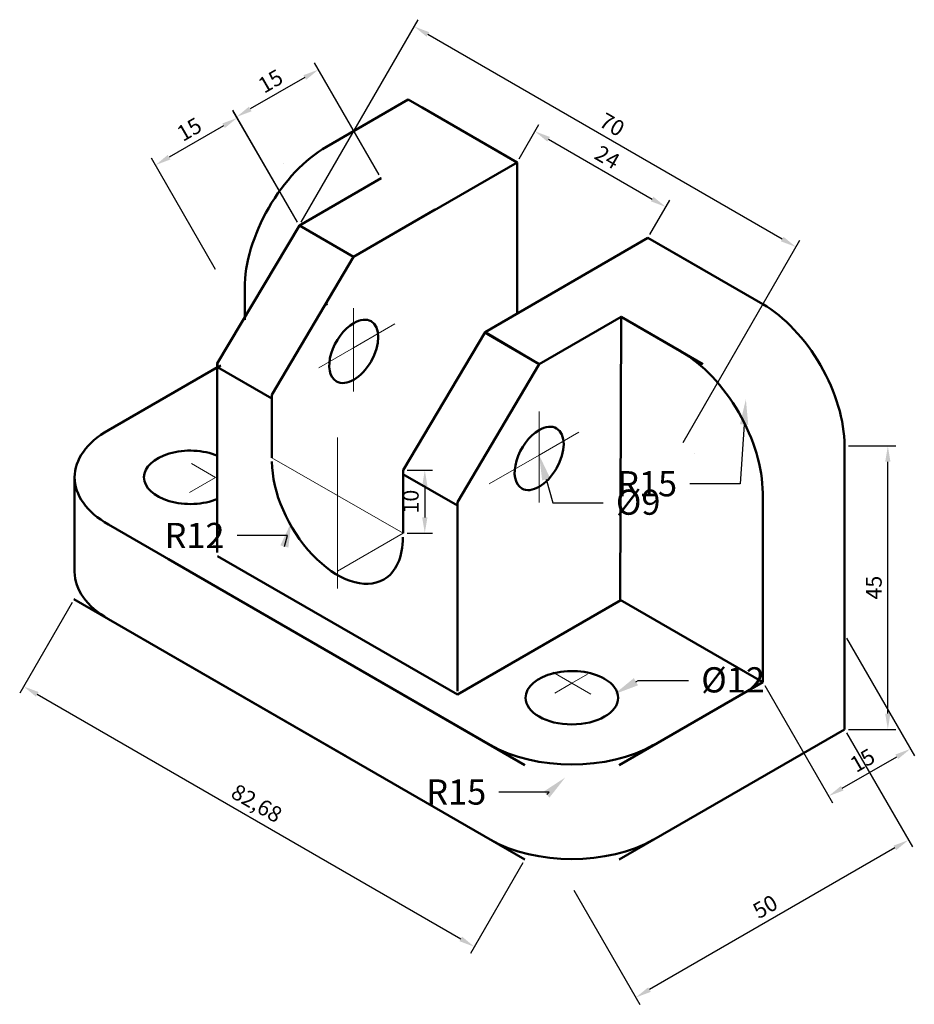
# Model space of a CAD drawing. Units: millimetres. Extents: x 2245 to 2387, y 1433 to 1590.
import ezdxf
from ezdxf import colors
from ezdxf.entities.mleader import LeaderData, LeaderLine
from ezdxf.math import Vec2, Vec3

# ---------------------------------------------------------------- set-up
doc = ezdxf.new("R2010")
doc.units = ezdxf.units.MM
doc.linetypes.add('CENTER', pattern=[50.8, 31.75, -6.35, 6.35, -6.35])
for name, color, linetype, lineweight in [('M-CNTR', 4, 'CENTER', 18), ('M-DIMS', 2, 'Continuous', 25), ('M-OUTL', 7, 'Continuous', 50)]:
    doc.layers.add(name, color=color, linetype=linetype, lineweight=lineweight)
doc.styles.get("Standard").update_dxf_attribs({"font": 'arial.ttf'})
doc.dimstyles.new('ISO-25', dxfattribs={"dimtxt": 2.5, "dimasz": 2.5, "dimexe": 1.25, "dimexo": 0.625, "dimtad": 1, "dimtxsty": 'Standard', "dimcen": 2.5, "dimadec": 0, "dimazin": 0, "dimtfac": 1, "dimtmove": 0, "dimatfit": 3, "dimfxl": 1, "dimarcsym": 0})

# ---------------------------------------------------------------- blocks, each defined once
blk = doc.blocks.new('*D1')
at = {"layer": 'Defpoints', "color": 0, "transparency": 16777216}
for p in [(2324.24, 1567.07), (2347.86, 1559.99), (2345.02, 1555.07)]:
    blk.add_point(p, dxfattribs=at)
at = {"layer": 'M-DIMS', "color": 0, "lineweight": -2, "transparency": 16777216}
for p, q in [((2324.55, 1567.61), (2327.7, 1573.07)), ((2329.24, 1570.74), (2345.69, 1561.24)), ((2345.33, 1555.61), (2348.48, 1561.07))]:
    blk.add_line(p, q, dxfattribs=at)
at = {"layer": 'M-DIMS', "color": 0, "transparency": 16777216}
for points in [[(2329.45, 1571.1), (2329.03, 1570.38), (2327.08, 1571.99)], [(2345.9, 1561.6), (2345.49, 1560.88), (2347.86, 1559.99)]]:
    blk.add_solid(points, dxfattribs=at)
at = {"layer": 'M-DIMS', "color": 0, "transparency": 16777216, "insert": (2338.41, 1567.62), "char_height": 2.5, "attachment_point": 5, "rotation": 330}
blk.add_mtext('24', dxfattribs=at)
blk = doc.blocks.new('*D2')
at = {"layer": 'Defpoints', "color": 0, "transparency": 16777216}
for p in [(2307.9, 1588.64), (2289.65, 1557.04), (2350.27, 1522.04)]:
    blk.add_point(p, dxfattribs=at)
at = {"layer": 'M-DIMS', "color": 0, "lineweight": -2, "transparency": 16777216}
for p, q in [((2289.96, 1557.58), (2308.52, 1589.73)), ((2366.35, 1554.89), (2310.06, 1587.39)), ((2350.59, 1522.58), (2369.14, 1554.73))]:
    blk.add_line(p, q, dxfattribs=at)
at = {"layer": 'M-DIMS', "color": 0, "transparency": 16777216}
for points in [[(2310.27, 1587.75), (2309.85, 1587.03), (2307.9, 1588.64)], [(2366.56, 1555.25), (2366.15, 1554.53), (2368.52, 1553.64)]]:
    blk.add_solid(points, dxfattribs=at)
at = {"layer": 'M-DIMS', "color": 0, "transparency": 16777216, "insert": (2339.16, 1572.79), "char_height": 2.5, "attachment_point": 5, "rotation": 330}
blk.add_mtext('70', dxfattribs=at)
blk = doc.blocks.new('*D3')
at = {"layer": 'Defpoints', "color": 0, "transparency": 16777216}
for p in [(2376.25, 1522.04), (2383.12, 1522.04), (2376.25, 1477.04)]:
    blk.add_point(p, dxfattribs=at)
at = {"layer": 'M-DIMS', "color": 0, "lineweight": -2, "transparency": 16777216}
for p, q in [((2376.88, 1522.04), (2384.37, 1522.04)), ((2383.12, 1479.54), (2383.12, 1519.54)), ((2376.88, 1477.04), (2384.37, 1477.04))]:
    blk.add_line(p, q, dxfattribs=at)
at = {"layer": 'M-DIMS', "color": 0, "transparency": 16777216}
for points in [[(2382.7, 1519.54), (2383.54, 1519.54), (2383.12, 1522.04)], [(2382.7, 1479.54), (2383.54, 1479.54), (2383.12, 1477.04)]]:
    blk.add_solid(points, dxfattribs=at)
at = {"layer": 'M-DIMS', "color": 0, "transparency": 16777216, "insert": (2381.22, 1499.54), "char_height": 2.5, "attachment_point": 5, "rotation": 90}
blk.add_mtext('45', dxfattribs=at)
blk = doc.blocks.new('*D4')
at = {"layer": 'Defpoints', "color": 0, "transparency": 16777216}
for p in [(2376.25, 1492.04), (2363.26, 1484.54), (2386.7, 1473.94)]:
    blk.add_point(p, dxfattribs=at)
at = {"layer": 'M-DIMS', "color": 0, "lineweight": -2, "transparency": 16777216}
for p, q in [((2376.57, 1491.5), (2387.33, 1472.86)), ((2363.58, 1484), (2374.34, 1465.36)), ((2375.88, 1467.69), (2384.54, 1472.69))]:
    blk.add_line(p, q, dxfattribs=at)
at = {"layer": 'M-DIMS', "color": 0, "transparency": 16777216}
for points in [[(2384.33, 1473.05), (2384.75, 1472.33), (2386.7, 1473.94)], [(2375.67, 1468.05), (2376.08, 1467.33), (2373.71, 1466.44)]]:
    blk.add_solid(points, dxfattribs=at)
at = {"layer": 'M-DIMS', "color": 0, "transparency": 16777216, "insert": (2379.26, 1471.84), "char_height": 2.5, "attachment_point": 5, "rotation": 30}
blk.add_mtext('15', dxfattribs=at)
blk = doc.blocks.new('*D5')
at = {"layer": 'Defpoints', "color": 0, "transparency": 16777216}
for p in [(2376.25, 1477.04), (2332.95, 1452.04), (2343.1, 1434.47)]:
    blk.add_point(p, dxfattribs=at)
at = {"layer": 'M-DIMS', "color": 0, "lineweight": -2, "transparency": 16777216}
for p, q in [((2376.57, 1476.5), (2387.02, 1458.38)), ((2384.23, 1458.22), (2345.26, 1435.72)), ((2333.26, 1451.5), (2343.72, 1433.38))]:
    blk.add_line(p, q, dxfattribs=at)
at = {"layer": 'M-DIMS', "color": 0, "transparency": 16777216}
for points in [[(2384.02, 1458.58), (2384.44, 1457.86), (2386.4, 1459.47)], [(2345.05, 1436.08), (2345.47, 1435.36), (2343.1, 1434.47)]]:
    blk.add_solid(points, dxfattribs=at)
at = {"layer": 'M-DIMS', "color": 0, "transparency": 16777216, "insert": (2363.8, 1448.61), "char_height": 2.5, "attachment_point": 5, "rotation": 30}
blk.add_mtext('50', dxfattribs=at)
blk = doc.blocks.new('*D6')
at = {"layer": 'Defpoints', "color": 0, "transparency": 16777216}
for p in [(2279.69, 1574.3), (2302.64, 1564.54), (2289.65, 1557.04)]:
    blk.add_point(p, dxfattribs=at)
at = {"layer": 'M-DIMS', "color": 0, "lineweight": -2, "transparency": 16777216}
for p, q in [((2302.33, 1565.08), (2292.05, 1582.88)), ((2290.51, 1580.55), (2281.85, 1575.55)), ((2289.34, 1557.58), (2279.06, 1575.38))]:
    blk.add_line(p, q, dxfattribs=at)
at = {"layer": 'M-DIMS', "color": 0, "transparency": 16777216}
for points in [[(2290.3, 1580.91), (2290.72, 1580.18), (2292.68, 1581.8)], [(2281.64, 1575.91), (2282.06, 1575.18), (2279.69, 1574.3)]]:
    blk.add_solid(points, dxfattribs=at)
at = {"layer": 'M-DIMS', "color": 0, "transparency": 16777216, "insert": (2285.23, 1579.69), "char_height": 2.5, "attachment_point": 5, "rotation": 30}
blk.add_mtext('15', dxfattribs=at)
blk = doc.blocks.new('*D7')
at = {"layer": 'Defpoints', "color": 0, "transparency": 16777216}
for p in [(2266.79, 1566.64), (2289.65, 1557.04), (2276.66, 1549.54)]:
    blk.add_point(p, dxfattribs=at)
at = {"layer": 'M-DIMS', "color": 0, "lineweight": -2, "transparency": 16777216}
for p, q in [((2289.34, 1557.58), (2279.15, 1575.22)), ((2277.61, 1572.89), (2268.95, 1567.89)), ((2276.35, 1550.08), (2266.16, 1567.72))]:
    blk.add_line(p, q, dxfattribs=at)
at = {"layer": 'M-DIMS', "color": 0, "transparency": 16777216}
for points in [[(2277.41, 1573.25), (2277.82, 1572.53), (2279.78, 1574.14)], [(2268.74, 1568.25), (2269.16, 1567.53), (2266.79, 1566.64)]]:
    blk.add_solid(points, dxfattribs=at)
at = {"layer": 'M-DIMS', "color": 0, "transparency": 16777216, "insert": (2272.33, 1572.04), "char_height": 2.5, "attachment_point": 5, "rotation": 30}
blk.add_mtext('15', dxfattribs=at)
blk = doc.blocks.new('*D8')
at = {"layer": 'Defpoints', "color": 0, "transparency": 16777216}
for p in [(2306.16, 1518.2), (2306.16, 1508.2), (2309.57, 1508.2)]:
    blk.add_point(p, dxfattribs=at)
at = {"layer": 'M-DIMS', "color": 0, "lineweight": -2, "transparency": 16777216}
for p, q in [((2306.79, 1518.2), (2310.82, 1518.2)), ((2309.57, 1515.7), (2309.57, 1510.7)), ((2306.79, 1508.2), (2310.82, 1508.2))]:
    blk.add_line(p, q, dxfattribs=at)
at = {"layer": 'M-DIMS', "color": 0, "transparency": 16777216}
for points in [[(2309.16, 1515.7), (2309.99, 1515.7), (2309.57, 1518.2)], [(2309.16, 1510.7), (2309.99, 1510.7), (2309.57, 1508.2)]]:
    blk.add_solid(points, dxfattribs=at)
at = {"layer": 'M-DIMS', "color": 0, "transparency": 16777216, "insert": (2307.67, 1513.2), "char_height": 2.5, "attachment_point": 5, "rotation": 90}
blk.add_mtext('10', dxfattribs=at)
blk = doc.blocks.new('*D9')
at = {"layer": 'Defpoints', "color": 0, "transparency": 16777216}
for p in [(2253.85, 1497.71), (2325.45, 1456.37), (2317.45, 1442.52)]:
    blk.add_point(p, dxfattribs=at)
at = {"layer": 'M-DIMS', "color": 0, "lineweight": -2, "transparency": 16777216}
for p, q in [((2253.54, 1497.17), (2245.23, 1482.77)), ((2248.02, 1482.61), (2315.29, 1443.77)), ((2325.14, 1455.83), (2316.83, 1441.43))]:
    blk.add_line(p, q, dxfattribs=at)
at = {"layer": 'M-DIMS', "color": 0, "transparency": 16777216}
for points in [[(2248.23, 1482.97), (2247.81, 1482.24), (2245.85, 1483.86)], [(2315.5, 1444.13), (2315.08, 1443.4), (2317.45, 1442.52)]]:
    blk.add_solid(points, dxfattribs=at)
at = {"layer": 'M-DIMS', "color": 0, "transparency": 16777216, "insert": (2282.72, 1465.03), "char_height": 2.5, "attachment_point": 5, "rotation": 330}
blk.add_mtext('82,68', dxfattribs=at)

msp = doc.modelspace()

# ---------------------------------------------------------------- linework, layer by layer
at = {"layer": 'M-CNTR'}
for p, q in [((2298.237, 1537.629), (2298.237, 1543.93)), ((2298.237, 1537.629), (2304.814, 1541.426)), ((2298.237, 1537.629), (2292.726, 1534.447)), ((2298.237, 1537.629), (2298.237, 1530.715)), ((2327.737, 1520.597), (2327.737, 1527.487)), ((2295.714, 1514.172), (2295.714, 1523.41)), ((2327.737, 1520.597), (2334.016, 1524.222)), ((2285.266, 1520.139), (2306.162, 1508.204)), ((2327.737, 1520.597), (2319.789, 1516.008)), ((2327.737, 1520.597), (2327.737, 1513.074)), ((2276.35, 1517.039), (2272.538, 1519.239)), ((2276.35, 1517.039), (2272.204, 1514.645)), ((2295.714, 1514.172), (2295.714, 1499.42)), ((2295.714, 1502.172), (2306.162, 1508.204)), ((2332.952, 1484.359), (2329.927, 1486.106)), ((2332.952, 1484.359), (2335.435, 1485.793)), ((2332.952, 1484.359), (2330.227, 1482.786)), ((2332.952, 1484.359), (2335.951, 1482.628))]:
    msp.add_line(p, q, dxfattribs=at)
at = {"layer": 'M-OUTL'}
for p, q in [((2306.954, 1577.062), (2293.963, 1569.562)), ((2306.954, 1577.062), (2324.274, 1567.062)), ((2324.237, 1567.07), (2309.15, 1575.781)), ((2324.237, 1567.07), (2319.962, 1569.539)), ((2287.175, 1566.872), (2287.175, 1566.872)), ((2324.237, 1567.07), (2308.992, 1558.269)), ((2324.237, 1567.07), (2324.237, 1543.07)), ((2302.641, 1564.539), (2289.651, 1557.039)), ((2302.641, 1564.539), (2302.586, 1564.57)), ((2311.246, 1559.57), (2298.256, 1552.07)), ((2311.246, 1559.57), (2298.256, 1552.07)), ((2276.605, 1535.139), (2289.651, 1557.039)), ((2298.256, 1552.07), (2289.651, 1557.039)), ((2293.981, 1554.539), (2289.651, 1557.039)), ((2319.152, 1540.135), (2345.021, 1555.07)), ((2363.263, 1544.539), (2345.021, 1555.07)), ((2353.737, 1550.039), (2345.021, 1555.07)), ((2353.737, 1550.039), (2345.021, 1555.07)), ((2298.256, 1552.07), (2285.266, 1530.139)), ((2280.973, 1547.062), (2280.973, 1542.062)), ((2293.698, 1544.375), (2294.137, 1544.628)), ((2340.746, 1542.539), (2327.756, 1535.039)), ((2340.63, 1497.606), (2340.746, 1542.539)), ((2350.273, 1537.039), (2340.746, 1542.539)), ((2340.746, 1542.539), (2353.737, 1535.039)), ((2340.746, 1542.539), (2343.345, 1541.039)), ((2340.746, 1542.539), (2343.345, 1541.039)), ((2319.152, 1540.135), (2306.162, 1518.204)), ((2327.756, 1535.039), (2319.095, 1540.039)), ((2327.756, 1535.039), (2319.152, 1540.135)), ((2327.756, 1535.039), (2319.152, 1540.135)), ((2324.237, 1537.123), (2324.237, 1537.07)), ((2259.322, 1524.562), (2276.643, 1534.562)), ((2268.85, 1530.029), (2277.153, 1534.823)), ((2268.85, 1530.029), (2277.153, 1534.823)), ((2276.605, 1535.139), (2276.605, 1513.278)), ((2276.605, 1505.139), (2276.605, 1535.139)), ((2285.303, 1529.562), (2276.643, 1534.562)), ((2276.661, 1534.539), (2276.661, 1535.232)), ((2314.766, 1513.108), (2327.756, 1535.039)), ((2285.266, 1530.139), (2285.266, 1520.139)), ((2376.254, 1477.039), (2376.254, 1522.039)), ((2352.396, 1520.813), (2352.396, 1520.813)), ((2306.162, 1518.204), (2306.162, 1508.204)), ((2253.941, 1502.062), (2253.941, 1517.062)), ((2314.748, 1512.562), (2306.088, 1517.562)), ((2363.263, 1514.539), (2363.263, 1484.539)), ((2276.605, 1513.278), (2276.605, 1505.139)), ((2314.766, 1483.108), (2314.766, 1513.108)), ((2314.766, 1513.108), (2314.766, 1483.108)), ((2319.944, 1474.562), (2259.322, 1509.562)), ((2268.85, 1504.048), (2325.452, 1471.369)), ((2314.748, 1482.562), (2276.643, 1504.562)), ((2297.151, 1472.708), (2253.85, 1497.708)), ((2314.748, 1482.562), (2340.729, 1497.562)), ((2363.263, 1484.539), (2340.63, 1497.606)), ((2268.85, 1489.048), (2325.452, 1456.369)), ((2340.452, 1471.369), (2363.263, 1484.539)), ((2340.452, 1456.369), (2376.254, 1477.039))]:
    msp.add_line(p, q, dxfattribs=at)
for centre, major_axis, start_param, end_param in [((2293.963, 1554.562), (-9.186, -15.91), 3.9269908, 5.4977872), ((2363.245, 1529.562), (9.186, -15.91), 0.7853981, 2.3561946), ((2298.293, 1537.062), (2.756, 4.773), 0.7853982, 3.1415927), ((2298.293, 1537.062), (2.756, 4.773), 3.1415927, 6.2831853), ((2298.293, 1537.062), (2.756, 4.773), 0, 0.7853982), ((2350.255, 1522.062), (9.186, -15.91), 0.7853981, 2.3561946), ((2272.313, 1517.062), (-18.371, 0), 5.4977871, 6.2831853), ((2327.738, 1520.062), (2.756, 4.773), 0.7853982, 3.1415927), ((2327.738, 1520.062), (2.756, 4.773), 3.1415927, 6.2831853), ((2327.738, 1520.062), (2.756, 4.773), 0, 0.7853982), ((2272.313, 1517.062), (7.348, 0), 0.9406591, 3.1415927), ((2295.695, 1513.562), (-7.348, 12.728), 0.7853982, 3.1415927), ((2272.313, 1517.062), (-18.371, 0), 0, 0.7853982), ((2272.313, 1517.062), (7.348, 0), 3.1415927, 5.3425262), ((2295.695, 1513.562), (-7.348, 12.728), 3.1415927, 3.9269908), ((2272.313, 1502.062), (-18.371, 0), 0, 0.7853982), ((2332.934, 1482.062), (7.348, 0), 0.7853982, 3.1415927), ((2332.934, 1482.062), (7.348, 0), 0, 0.7853982), ((2332.934, 1482.062), (7.348, 0), 3.1415927, 6.2831853), ((2332.934, 1482.062), (18.371, 0), 3.9269908, 5.4977871), ((2332.934, 1467.062), (18.371, 0), 3.9269908, 5.4977871)]:
    msp.add_ellipse(centre, major_axis=major_axis, ratio=0.5773503, start_param=start_param, end_param=end_param, dxfattribs=at)

# ---------------------------------------------------------------- dimensions: what is measured, and where the dimension line sits
at = {"layer": 'M-DIMS'}
for p1, p2, distance, picture, middle in [((2350.273, 1522.039), (2289.651, 1557.039), -36.494, '*D2', (2339.16, 1572.79)), ((2302.641, 1564.539), (2289.651, 1557.039), -19.926, '*D6', (2285.232, 1579.692)), ((2289.651, 1557.039), (2276.661, 1549.539), -19.745, '*D7', (2272.333, 1572.035)), ((2324.237, 1567.07), (2345.021, 1555.07), 5.677, '*D1', (2338.408, 1567.615)), ((2376.254, 1477.039), (2376.254, 1522.039), -6.868, '*D3', (2381.225, 1499.539)), ((2306.162, 1518.204), (2306.162, 1508.204), 3.41, '*D8', (2307.67, 1513.204)), ((2363.263, 1484.539), (2376.254, 1492.039), -20.897, '*D4', (2379.256, 1471.838)), ((2376.254, 1477.039), (2332.952, 1452.039), 20.29, '*D5', (2363.797, 1448.614))]:
    dim = msp.add_aligned_dim(p1=p1, p2=p2, distance=distance, dimstyle='ISO-25', override={"dimclrd": 0, "dimclre": 0, "dimclrt": 0}, dxfattribs=at)
    dim.commit()
    dim.dimension.update_dxf_attribs({"geometry": picture, "text_midpoint": middle})
dim = msp.add_linear_dim(base=(2317.454, 1442.516), p1=(2253.85, 1497.708), p2=(2325.452, 1456.369), angle=330, dimstyle='ISO-25', override={"dimrnd": 0}, dxfattribs=at)
dim.commit()
dim.dimension.update_dxf_attribs({"geometry": '*D9', "text_midpoint": (2282.717, 1465.028)})

# ---------------------------------------------------------------- leaders
ml = msp.add_multileader_mtext('Standard', dxfattribs=at)
ml.set_content('R15', color=256)
ml.set_leader_properties()
ml.build(insert=Vec2(0, 0))
ctx = ml.context
ctx.base_point, ctx.plane_origin = Vec3(2338.057, 1516.008), Vec3(2360.571, 1529.452)
ctx.text_align_type = 2
notes = []
notes.append((ctx, [(0, (1, 1, 0), (2359.645, 1516.008), (-1, 0), 8, [(0, [(2360.571, 1529.452)], 0, [])])]))
ctx.mtext.insert, ctx.mtext.alignment, ctx.mtext.flow_direction = Vec3(2349.645, 1518.042), 3, 5
ml = msp.add_multileader_mtext('Standard', dxfattribs=at)
ml.set_content('Ø9', color=256)
ml.set_leader_properties()
ml.build(insert=Vec2(0, 0))
ctx = ml.context
ctx.base_point, ctx.plane_origin = Vec3(2337.925, 1513.037), Vec3(2327.737, 1520.597)
notes.append((ctx, [(0, (1, 1, 0), (2329.925, 1513.037), (1, 0), 8, [(0, [(2327.737, 1520.597)], 0, [])])]))
ctx.mtext.insert, ctx.mtext.flow_direction = Vec3(2339.925, 1515.118), 5
ml = msp.add_multileader_mtext('Standard', dxfattribs=at)
ml.set_content('R12', color=256)
ml.set_leader_properties()
ml.build(insert=Vec2(0, 0))
ctx = ml.context
ctx.base_point, ctx.plane_origin = Vec3(2266.249, 1507.829), Vec3(2288.365, 1509.929)
ctx.text_align_type = 2
notes.append((ctx, [(0, (1, 1, 0), (2287.766, 1507.829), (-1, 0), 8, [(0, [(2288.365, 1509.929)], 0, [])])]))
ctx.mtext.insert, ctx.mtext.alignment, ctx.mtext.flow_direction = Vec3(2277.766, 1509.829), 3, 5
ml = msp.add_multileader_mtext('Standard', dxfattribs=at)
ml.set_content('Ø12', color=256)
ml.set_leader_properties()
ml.build(insert=Vec2(0, 0))
ctx = ml.context
ctx.base_point, ctx.plane_origin = Vec3(2351.481, 1484.821), Vec3(2339.643, 1482.605)
notes.append((ctx, [(0, (1, 1, 0), (2343.481, 1484.821), (1, 0), 8, [(0, [(2339.643, 1482.605)], 0, [])])]))
ctx.mtext.insert, ctx.mtext.flow_direction = Vec3(2353.481, 1486.901), 5
ml = msp.add_multileader_mtext('Standard', dxfattribs=at)
ml.set_content('R15', color=256)
ml.set_leader_properties()
ml.build(insert=Vec2(0, 0))
ctx = ml.context
ctx.base_point, ctx.plane_origin = Vec3(2307.74, 1467.06), Vec3(2331.884, 1469.397)
ctx.text_align_type = 2
notes.append((ctx, [(0, (1, 1, 0), (2329.328, 1467.06), (-1, 0), 8, [(0, [(2331.884, 1469.397)], 0, [])])]))
ctx.mtext.insert, ctx.mtext.alignment, ctx.mtext.flow_direction = Vec3(2319.328, 1469.094), 3, 5
for ctx, leaders in notes:
    for number, flags, end, landing, length, lines in leaders:
        leader = LeaderData()
        leader.index, (leader.has_last_leader_line, leader.has_dogleg_vector, leader.attachment_direction) = number, flags
        leader.last_leader_point, leader.dogleg_vector, leader.dogleg_length = Vec3(end), Vec3(landing), length
        for number, points, colour, breaks in lines:
            line = LeaderLine()
            line.index, line.vertices, line.color, line.breaks = number, Vec3.list(points), colors.encode_raw_color(colour), breaks
            leader.lines.append(line)
        ctx.leaders.append(leader)

doc.saveas('drawing.dxf')
